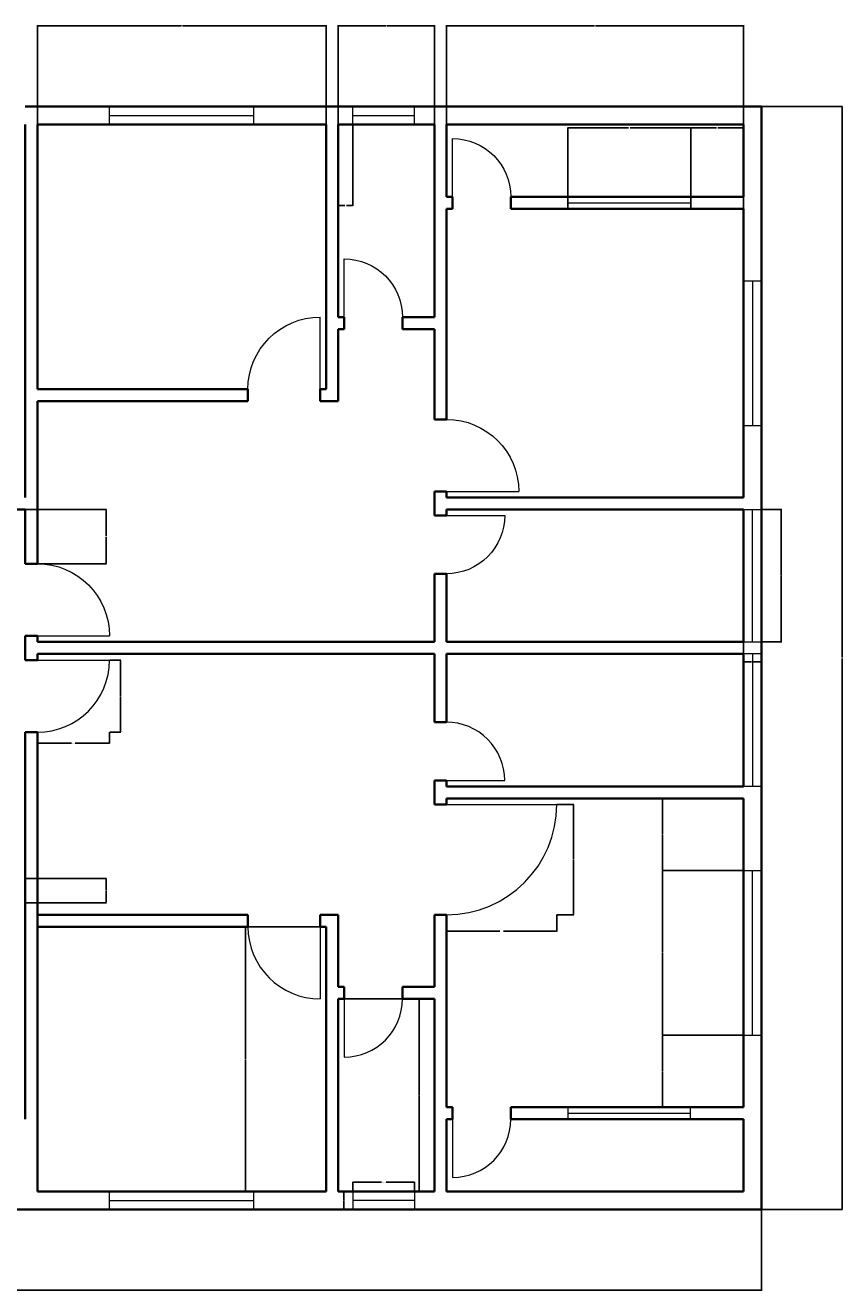
# Model space of a CAD drawing. Units: inches. Extents: x 2811 to 3694, y 2039 to 2670.
# Tile 3 of 3: x 3286 to 3694, y 2039 to 2670. Entities that reach past the tile are written whole.
import ezdxf

# ---------------------------------------------------------------- set-up
doc = ezdxf.new("R2010")
doc.units = ezdxf.units.IN
for name, color, linetype, lineweight in [('A-ANNO-DIMS', 2, 'Continuous', 18), ('A-DOOR', 3, 'Continuous', 18), ('A-GLAZ', 4, 'Continuous', 18), ('A-WALL', 7, 'Continuous', 35)]:
    doc.layers.add(name, color=color, linetype=linetype, lineweight=lineweight)
doc.styles.get("Standard").update_dxf_attribs({"font": 'arial.ttf'})
doc.dimstyles.get("Standard").update_dxf_attribs({"dimtxt": 0.18, "dimasz": 0.18, "dimexe": 0.18, "dimexo": 0.0625, "dimgap": 0.09, "dimtad": 0, "dimtih": 1, "dimtoh": 1, "dimdec": 4, "dimzin": 0, "dimdsep": 46, "dimtxsty": 'Standard', "dimcen": 0.09, "dimadec": 0, "dimazin": 0, "dimtfac": 1, "dimtdec": 4, "dimtofl": 0, "dimtmove": 0, "dimatfit": 3, "dimfxl": 1, "dimtolj": 1, "dimtzin": 0, "dimarcsym": 0})

# ---------------------------------------------------------------- blocks, each defined once
blk = doc.blocks.new('DOOR-SWING-29IN')
blk.add_line((29, 0), (29, 29))
blk.add_arc((29, 0), 29, 90, 180)
blk = doc.blocks.new('DOOR-SWING-36IN')
blk.add_line((36, 0), (0, 0))
blk.add_arc((36, 0), 36, 90, 180)
blk = doc.blocks.new('DOOR-SWING-55IN')
blk.add_line((0, 55), (55, 55))
blk.add_arc((0, 55), 55, 270, 0)
blk = doc.blocks.new('WIN-72IN')
for p, q in [((0, 0), (0, 9)), ((72, 0), (72, 9)), ((0, 4.5), (72, 4.5))]:
    blk.add_line(p, q)
blk = doc.blocks.new('WIN-66IN')
for p, q in [((0, 66), (9, 66)), ((4.5, 0), (4.5, 66)), ((0, 0), (9, 0))]:
    blk.add_line(p, q)
blk = doc.blocks.new('WIN-30_67IN')
for p, q in [((0, 0), (0, 9)), ((30.67, 0), (30.67, 9)), ((0, 4.5), (30.67, 4.5))]:
    blk.add_line(p, q)
blk = doc.blocks.new('*D10')
at = {"layer": 'A-ANNO-DIMS', "color": 0, "lineweight": -2, "transparency": 16777216}
for p, q in [((3292.28, 2317.92), (3292.28, 2312.4)), ((3328.28, 2317.92), (3328.28, 2312.4)), ((3292.46, 2312.58), (3309.34, 2312.58)), ((3328.1, 2312.58), (3311.21, 2312.58))]:
    blk.add_line(p, q, dxfattribs=at)
at = {"layer": 'A-ANNO-DIMS', "color": 0, "transparency": 16777216}
for points in [[(3292.46, 2312.61), (3292.46, 2312.55), (3292.28, 2312.58)], [(3328.1, 2312.61), (3328.1, 2312.55), (3328.28, 2312.58)]]:
    blk.add_solid(points, dxfattribs=at)
at = {"layer": 'Defpoints', "color": 0, "transparency": 16777216}
for p in [(3292.28, 2317.98), (3328.28, 2317.98), (3292.28, 2312.58)]:
    blk.add_point(p, dxfattribs=at)
at = {"layer": 'A-ANNO-DIMS', "color": 0, "transparency": 16777216, "insert": (3310.28, 2312.58), "char_height": 0.18, "attachment_point": 5}
blk.add_mtext('\\A1;DOOR 36 TYP.', dxfattribs=at)
blk = doc.blocks.new('*D11')
at = {"layer": 'A-ANNO-DIMS', "color": 0, "lineweight": -2, "transparency": 16777216}
for p, q in [((3328.34, 2353.98), (3333.86, 2353.98)), ((3333.68, 2353.8), (3333.68, 2336.16)), ((3333.68, 2318.16), (3333.68, 2335.8)), ((3328.34, 2317.98), (3333.86, 2317.98))]:
    blk.add_line(p, q, dxfattribs=at)
at = {"layer": 'A-ANNO-DIMS', "color": 0, "transparency": 16777216}
for points in [[(3333.65, 2353.8), (3333.71, 2353.8), (3333.68, 2353.98)], [(3333.65, 2318.16), (3333.71, 2318.16), (3333.68, 2317.98)]]:
    blk.add_solid(points, dxfattribs=at)
at = {"layer": 'Defpoints', "color": 0, "transparency": 16777216}
for p in [(3328.28, 2353.98), (3328.28, 2317.98), (3333.68, 2317.98)]:
    blk.add_point(p, dxfattribs=at)
at = {"layer": 'A-ANNO-DIMS', "color": 0, "transparency": 16777216, "insert": (3333.68, 2335.98), "char_height": 0.18, "attachment_point": 5}
blk.add_mtext('\\A1;36 TYP.', dxfattribs=at)
blk = doc.blocks.new('*D12')
at = {"layer": 'A-ANNO-DIMS', "color": 0, "lineweight": -2, "transparency": 16777216}
for p, q in [((3496.28, 2226.92), (3496.28, 2218.55)), ((3551.28, 2226.92), (3551.28, 2218.55)), ((3496.46, 2218.73), (3522.84, 2218.73)), ((3551.1, 2218.73), (3524.71, 2218.73))]:
    blk.add_line(p, q, dxfattribs=at)
at = {"layer": 'A-ANNO-DIMS', "color": 0, "transparency": 16777216}
for points in [[(3496.46, 2218.76), (3496.46, 2218.7), (3496.28, 2218.73)], [(3551.1, 2218.76), (3551.1, 2218.7), (3551.28, 2218.73)]]:
    blk.add_solid(points, dxfattribs=at)
at = {"layer": 'Defpoints', "color": 0, "transparency": 16777216}
for p in [(3496.28, 2226.98), (3551.28, 2226.98), (3551.28, 2218.73)]:
    blk.add_point(p, dxfattribs=at)
at = {"layer": 'A-ANNO-DIMS', "color": 0, "transparency": 16777216, "insert": (3523.78, 2218.73), "char_height": 0.18, "attachment_point": 5}
blk.add_mtext('\\A1;DOOR 55 TYP.', dxfattribs=at)
blk = doc.blocks.new('*D13')
at = {"layer": 'A-ANNO-DIMS', "color": 0, "lineweight": -2, "transparency": 16777216}
for p, q in [((3551.34, 2281.98), (3559.71, 2281.98)), ((3559.53, 2281.8), (3559.53, 2254.66)), ((3559.53, 2227.16), (3559.53, 2254.3)), ((3551.34, 2226.98), (3559.71, 2226.98))]:
    blk.add_line(p, q, dxfattribs=at)
at = {"layer": 'A-ANNO-DIMS', "color": 0, "transparency": 16777216}
for points in [[(3559.5, 2281.8), (3559.56, 2281.8), (3559.53, 2281.98)], [(3559.5, 2227.16), (3559.56, 2227.16), (3559.53, 2226.98)]]:
    blk.add_solid(points, dxfattribs=at)
at = {"layer": 'Defpoints', "color": 0, "transparency": 16777216}
for p in [(3551.28, 2281.98), (3559.53, 2281.98), (3551.28, 2226.98)]:
    blk.add_point(p, dxfattribs=at)
at = {"layer": 'A-ANNO-DIMS', "color": 0, "transparency": 16777216, "insert": (3559.53, 2254.48), "char_height": 0.18, "attachment_point": 5}
blk.add_mtext('\\A1;55 TYP.', dxfattribs=at)
blk = doc.blocks.new('*D16')
at = {"layer": 'A-ANNO-DIMS', "color": 0, "lineweight": -2, "transparency": 16777216}
for p, q in [((3653.34, 2428.98), (3663.36, 2428.98)), ((3663.18, 2428.8), (3663.18, 2396.16)), ((3663.18, 2363.16), (3663.18, 2395.8)), ((3653.34, 2362.98), (3663.36, 2362.98))]:
    blk.add_line(p, q, dxfattribs=at)
at = {"layer": 'A-ANNO-DIMS', "color": 0, "transparency": 16777216}
for points in [[(3663.15, 2428.8), (3663.21, 2428.8), (3663.18, 2428.98)], [(3663.15, 2363.16), (3663.21, 2363.16), (3663.18, 2362.98)]]:
    blk.add_solid(points, dxfattribs=at)
at = {"layer": 'Defpoints', "color": 0, "transparency": 16777216}
for p in [(3653.28, 2428.98), (3663.18, 2428.98), (3653.28, 2362.98)]:
    blk.add_point(p, dxfattribs=at)
at = {"layer": 'A-ANNO-DIMS', "color": 0, "transparency": 16777216, "insert": (3663.18, 2395.98), "char_height": 0.18, "attachment_point": 5}
blk.add_mtext('\\A1;WINDOW 66 TYP.', dxfattribs=at)
blk = doc.blocks.new('*D17')
at = {"layer": 'A-ANNO-DIMS', "color": 0, "lineweight": -2, "transparency": 16777216}
for p, q in [((3644.28, 2362.92), (3644.28, 2352.9)), ((3653.28, 2362.92), (3653.28, 2352.9)), ((3644.46, 2353.08), (3648.32, 2353.08)), ((3653.1, 2353.08), (3649.23, 2353.08))]:
    blk.add_line(p, q, dxfattribs=at)
at = {"layer": 'A-ANNO-DIMS', "color": 0, "transparency": 16777216}
for points in [[(3644.46, 2353.11), (3644.46, 2353.05), (3644.28, 2353.08)], [(3653.1, 2353.11), (3653.1, 2353.05), (3653.28, 2353.08)]]:
    blk.add_solid(points, dxfattribs=at)
at = {"layer": 'Defpoints', "color": 0, "transparency": 16777216}
for p in [(3644.28, 2362.98), (3653.28, 2362.98), (3653.28, 2353.08)]:
    blk.add_point(p, dxfattribs=at)
at = {"layer": 'A-ANNO-DIMS', "color": 0, "transparency": 16777216, "insert": (3648.78, 2353.08), "char_height": 0.18, "attachment_point": 5}
blk.add_mtext('\\A1;9 TYP.', dxfattribs=at)
blk = doc.blocks.new('*D20')
at = {"layer": 'A-ANNO-DIMS', "color": 0, "lineweight": -2, "transparency": 16777216}
for p, q in [((3449.64, 2089.04), (3449.64, 2093.76)), ((3449.82, 2093.58), (3463.86, 2093.58)), ((3480.13, 2093.58), (3466.1, 2093.58)), ((3480.31, 2089.04), (3480.31, 2093.76))]:
    blk.add_line(p, q, dxfattribs=at)
at = {"layer": 'A-ANNO-DIMS', "color": 0, "transparency": 16777216}
for points in [[(3449.82, 2093.61), (3449.82, 2093.55), (3449.64, 2093.58)], [(3480.13, 2093.61), (3480.13, 2093.55), (3480.31, 2093.58)]]:
    blk.add_solid(points, dxfattribs=at)
at = {"layer": 'Defpoints', "color": 0, "transparency": 16777216}
for p in [(3449.64, 2093.58), (3449.64, 2088.98), (3480.31, 2088.98)]:
    blk.add_point(p, dxfattribs=at)
at = {"layer": 'A-ANNO-DIMS', "color": 0, "transparency": 16777216, "insert": (3464.98, 2093.58), "char_height": 0.18, "attachment_point": 5}
blk.add_mtext('\\A1;WINDOW 31 TYP.', dxfattribs=at)
blk = doc.blocks.new('*D21')
at = {"layer": 'A-ANNO-DIMS', "color": 0, "lineweight": -2, "transparency": 16777216}
for p, q in [((3449.58, 2088.98), (3444.86, 2088.98)), ((3445.04, 2088.8), (3445.04, 2084.66)), ((3445.04, 2080.16), (3445.04, 2084.3)), ((3449.58, 2079.98), (3444.86, 2079.98))]:
    blk.add_line(p, q, dxfattribs=at)
at = {"layer": 'A-ANNO-DIMS', "color": 0, "transparency": 16777216}
for points in [[(3445.01, 2088.8), (3445.07, 2088.8), (3445.04, 2088.98)], [(3445.01, 2080.16), (3445.07, 2080.16), (3445.04, 2079.98)]]:
    blk.add_solid(points, dxfattribs=at)
at = {"layer": 'Defpoints', "color": 0, "transparency": 16777216}
for p in [(3449.64, 2088.98), (3445.04, 2079.98), (3449.64, 2079.98)]:
    blk.add_point(p, dxfattribs=at)
at = {"layer": 'A-ANNO-DIMS', "color": 0, "transparency": 16777216, "insert": (3445.04, 2084.48), "char_height": 0.18, "attachment_point": 5}
blk.add_mtext('\\A1;9 TYP.', dxfattribs=at)
blk = doc.blocks.new('*D22')
at = {"layer": 'A-ANNO-DIMS', "color": 0, "lineweight": -2, "transparency": 16777216}
for p, q in [((2851.28, 2079.92), (2851.28, 2039.5)), ((3653.28, 2079.92), (3653.28, 2039.5)), ((2851.46, 2039.68), (3251.99, 2039.68)), ((3653.1, 2039.68), (3252.56, 2039.68))]:
    blk.add_line(p, q, dxfattribs=at)
at = {"layer": 'A-ANNO-DIMS', "color": 0, "transparency": 16777216}
for points in [[(2851.46, 2039.71), (2851.46, 2039.65), (2851.28, 2039.68)], [(3653.1, 2039.71), (3653.1, 2039.65), (3653.28, 2039.68)]]:
    blk.add_solid(points, dxfattribs=at)
at = {"layer": 'Defpoints', "color": 0, "transparency": 16777216}
for p in [(2851.28, 2079.98), (3653.28, 2079.98), (3653.28, 2039.68)]:
    blk.add_point(p, dxfattribs=at)
at = {"layer": 'A-ANNO-DIMS', "color": 0, "transparency": 16777216, "insert": (3252.28, 2039.68), "char_height": 0.18, "attachment_point": 5}
blk.add_mtext('\\A1;802', dxfattribs=at)
blk = doc.blocks.new('*D23')
at = {"layer": 'A-ANNO-DIMS', "color": 0, "lineweight": -2, "transparency": 16777216}
for p, q in [((3653.34, 2629.98), (3693.76, 2629.98)), ((3693.58, 2629.8), (3693.58, 2355.16)), ((3693.58, 2080.16), (3693.58, 2354.8)), ((3653.34, 2079.98), (3693.76, 2079.98))]:
    blk.add_line(p, q, dxfattribs=at)
at = {"layer": 'A-ANNO-DIMS', "color": 0, "transparency": 16777216}
for points in [[(3693.55, 2629.8), (3693.61, 2629.8), (3693.58, 2629.98)], [(3693.55, 2080.16), (3693.61, 2080.16), (3693.58, 2079.98)]]:
    blk.add_solid(points, dxfattribs=at)
at = {"layer": 'Defpoints', "color": 0, "transparency": 16777216}
for p in [(3653.28, 2629.98), (3693.58, 2629.98), (3653.28, 2079.98)]:
    blk.add_point(p, dxfattribs=at)
at = {"layer": 'A-ANNO-DIMS', "color": 0, "transparency": 16777216, "insert": (3693.58, 2354.98), "char_height": 0.18, "attachment_point": 5}
blk.add_mtext('\\A1;550', dxfattribs=at)
blk = doc.blocks.new('*D28')
at = {"layer": 'A-ANNO-DIMS', "color": 0, "lineweight": -2, "transparency": 16777216}
for p, q in [((3292.28, 2621.04), (3292.28, 2670.46)), ((3292.46, 2670.28), (3364, 2670.28)), ((3436.1, 2670.28), (3364.56, 2670.28)), ((3436.28, 2621.04), (3436.28, 2670.46))]:
    blk.add_line(p, q, dxfattribs=at)
at = {"layer": 'A-ANNO-DIMS', "color": 0, "transparency": 16777216}
for points in [[(3292.46, 2670.31), (3292.46, 2670.25), (3292.28, 2670.28)], [(3436.1, 2670.31), (3436.1, 2670.25), (3436.28, 2670.28)]]:
    blk.add_solid(points, dxfattribs=at)
at = {"layer": 'Defpoints', "color": 0, "transparency": 16777216}
for p in [(3436.28, 2670.28), (3292.28, 2620.98), (3436.28, 2620.98)]:
    blk.add_point(p, dxfattribs=at)
at = {"layer": 'A-ANNO-DIMS', "color": 0, "transparency": 16777216, "insert": (3364.28, 2670.28), "char_height": 0.18, "attachment_point": 5}
blk.add_mtext('\\A1;144', dxfattribs=at)
blk = doc.blocks.new('*D29')
at = {"layer": 'A-ANNO-DIMS', "color": 0, "lineweight": -2, "transparency": 16777216}
for p, q in [((3442.28, 2621.04), (3442.28, 2670.46)), ((3442.46, 2670.28), (3466.05, 2670.28)), ((3490.1, 2670.28), (3466.5, 2670.28)), ((3490.28, 2621.04), (3490.28, 2670.46))]:
    blk.add_line(p, q, dxfattribs=at)
at = {"layer": 'A-ANNO-DIMS', "color": 0, "transparency": 16777216}
for points in [[(3442.46, 2670.31), (3442.46, 2670.25), (3442.28, 2670.28)], [(3490.1, 2670.31), (3490.1, 2670.25), (3490.28, 2670.28)]]:
    blk.add_solid(points, dxfattribs=at)
at = {"layer": 'Defpoints', "color": 0, "transparency": 16777216}
for p in [(3490.28, 2670.28), (3442.28, 2620.98), (3490.28, 2620.98)]:
    blk.add_point(p, dxfattribs=at)
at = {"layer": 'A-ANNO-DIMS', "color": 0, "transparency": 16777216, "insert": (3466.28, 2670.28), "char_height": 0.18, "attachment_point": 5}
blk.add_mtext('\\A1;48', dxfattribs=at)
blk = doc.blocks.new('*D30')
at = {"layer": 'A-ANNO-DIMS', "color": 0, "lineweight": -2, "transparency": 16777216}
for p, q in [((3496.28, 2621.04), (3496.28, 2670.46)), ((3496.46, 2670.28), (3570, 2670.28)), ((3644.1, 2670.28), (3570.56, 2670.28)), ((3644.28, 2621.04), (3644.28, 2670.46))]:
    blk.add_line(p, q, dxfattribs=at)
at = {"layer": 'A-ANNO-DIMS', "color": 0, "transparency": 16777216}
for points in [[(3496.46, 2670.31), (3496.46, 2670.25), (3496.28, 2670.28)], [(3644.1, 2670.31), (3644.1, 2670.25), (3644.28, 2670.28)]]:
    blk.add_solid(points, dxfattribs=at)
at = {"layer": 'Defpoints', "color": 0, "transparency": 16777216}
for p in [(3644.28, 2670.28), (3496.28, 2620.98), (3644.28, 2620.98)]:
    blk.add_point(p, dxfattribs=at)
at = {"layer": 'A-ANNO-DIMS', "color": 0, "transparency": 16777216, "insert": (3570.28, 2670.28), "char_height": 0.18, "attachment_point": 5}
blk.add_mtext('\\A1;148', dxfattribs=at)
blk = doc.blocks.new('*D42')
at = {"layer": 'A-ANNO-DIMS', "color": 0, "lineweight": -2, "transparency": 16777216}
for p, q in [((3436.21, 2220.98), (3395.8, 2220.98)), ((3395.98, 2220.8), (3395.98, 2155.16)), ((3395.98, 2089.16), (3395.98, 2154.8)), ((3436.21, 2088.98), (3395.8, 2088.98))]:
    blk.add_line(p, q, dxfattribs=at)
at = {"layer": 'A-ANNO-DIMS', "color": 0, "transparency": 16777216}
for points in [[(3395.95, 2220.8), (3396.01, 2220.8), (3395.98, 2220.98)], [(3395.95, 2089.16), (3396.01, 2089.16), (3395.98, 2088.98)]]:
    blk.add_solid(points, dxfattribs=at)
at = {"layer": 'Defpoints', "color": 0, "transparency": 16777216}
for p in [(3395.98, 2220.98), (3436.28, 2220.98), (3436.28, 2088.98)]:
    blk.add_point(p, dxfattribs=at)
at = {"layer": 'A-ANNO-DIMS', "color": 0, "transparency": 16777216, "insert": (3395.98, 2154.98), "char_height": 0.18, "attachment_point": 5}
blk.add_mtext('\\A1;132', dxfattribs=at)
blk = doc.blocks.new('*D43')
at = {"layer": 'A-ANNO-DIMS', "color": 0, "lineweight": -2, "transparency": 16777216}
for p, q in [((3442.34, 2184.98), (3482.76, 2184.98)), ((3482.58, 2184.8), (3482.58, 2137.16)), ((3482.58, 2089.16), (3482.58, 2136.8)), ((3442.34, 2088.98), (3482.76, 2088.98))]:
    blk.add_line(p, q, dxfattribs=at)
at = {"layer": 'A-ANNO-DIMS', "color": 0, "transparency": 16777216}
for points in [[(3482.55, 2184.8), (3482.61, 2184.8), (3482.58, 2184.98)], [(3482.55, 2089.16), (3482.61, 2089.16), (3482.58, 2088.98)]]:
    blk.add_solid(points, dxfattribs=at)
at = {"layer": 'Defpoints', "color": 0, "transparency": 16777216}
for p in [(3442.28, 2184.98), (3442.28, 2088.98), (3482.58, 2088.98)]:
    blk.add_point(p, dxfattribs=at)
at = {"layer": 'A-ANNO-DIMS', "color": 0, "transparency": 16777216, "insert": (3482.58, 2136.98), "char_height": 0.18, "attachment_point": 5}
blk.add_mtext('\\A1;96', dxfattribs=at)
blk = doc.blocks.new('*D44')
at = {"layer": 'A-ANNO-DIMS', "color": 0, "lineweight": -2, "transparency": 16777216}
for p, q in [((3644.21, 2248.98), (3603.8, 2248.98)), ((3603.98, 2248.8), (3603.98, 2208.16)), ((3603.98, 2167.16), (3603.98, 2207.8)), ((3644.21, 2166.98), (3603.8, 2166.98))]:
    blk.add_line(p, q, dxfattribs=at)
at = {"layer": 'A-ANNO-DIMS', "color": 0, "transparency": 16777216}
for points in [[(3603.95, 2248.8), (3604.01, 2248.8), (3603.98, 2248.98)], [(3603.95, 2167.16), (3604.01, 2167.16), (3603.98, 2166.98)]]:
    blk.add_solid(points, dxfattribs=at)
at = {"layer": 'Defpoints', "color": 0, "transparency": 16777216}
for p in [(3603.98, 2248.98), (3644.28, 2248.98), (3644.28, 2166.98)]:
    blk.add_point(p, dxfattribs=at)
at = {"layer": 'A-ANNO-DIMS', "color": 0, "transparency": 16777216, "insert": (3603.98, 2207.98), "char_height": 0.18, "attachment_point": 5}
blk.add_mtext('\\A1;82', dxfattribs=at)
blk = doc.blocks.new('*D45')
at = {"layer": 'A-ANNO-DIMS', "color": 0, "lineweight": -2, "transparency": 16777216}
for p, q in [((3644.21, 2166.98), (3603.8, 2166.98)), ((3603.98, 2166.8), (3603.98, 2149.16)), ((3603.98, 2131.16), (3603.98, 2148.8)), ((3644.21, 2130.98), (3603.8, 2130.98))]:
    blk.add_line(p, q, dxfattribs=at)
at = {"layer": 'A-ANNO-DIMS', "color": 0, "transparency": 16777216}
for points in [[(3603.95, 2166.8), (3604.01, 2166.8), (3603.98, 2166.98)], [(3603.95, 2131.16), (3604.01, 2131.16), (3603.98, 2130.98)]]:
    blk.add_solid(points, dxfattribs=at)
at = {"layer": 'Defpoints', "color": 0, "transparency": 16777216}
for p in [(3603.98, 2166.98), (3644.28, 2166.98), (3644.28, 2130.98)]:
    blk.add_point(p, dxfattribs=at)
at = {"layer": 'A-ANNO-DIMS', "color": 0, "transparency": 16777216, "insert": (3603.98, 2148.98), "char_height": 0.18, "attachment_point": 5}
blk.add_mtext('\\A1;36', dxfattribs=at)
blk = doc.blocks.new('*D46')
at = {"layer": 'A-ANNO-DIMS', "color": 0, "lineweight": -2, "transparency": 16777216}
for p, q in [((3644.21, 2284.98), (3603.8, 2284.98)), ((3603.98, 2284.8), (3603.98, 2267.16)), ((3603.98, 2249.16), (3603.98, 2266.8)), ((3644.21, 2248.98), (3603.8, 2248.98))]:
    blk.add_line(p, q, dxfattribs=at)
at = {"layer": 'A-ANNO-DIMS', "color": 0, "transparency": 16777216}
for points in [[(3603.95, 2284.8), (3604.01, 2284.8), (3603.98, 2284.98)], [(3603.95, 2249.16), (3604.01, 2249.16), (3603.98, 2248.98)]]:
    blk.add_solid(points, dxfattribs=at)
at = {"layer": 'Defpoints', "color": 0, "transparency": 16777216}
for p in [(3603.98, 2284.98), (3644.28, 2284.98), (3644.28, 2248.98)]:
    blk.add_point(p, dxfattribs=at)
at = {"layer": 'A-ANNO-DIMS', "color": 0, "transparency": 16777216, "insert": (3603.98, 2266.98), "char_height": 0.18, "attachment_point": 5}
blk.add_mtext('\\A1;36', dxfattribs=at)
blk = doc.blocks.new('*D49')
at = {"layer": 'A-ANNO-DIMS', "color": 0, "lineweight": -2, "transparency": 16777216}
for p, q in [((3556.69, 2579.04), (3556.69, 2619.46)), ((3556.87, 2619.28), (3587.02, 2619.28)), ((3617.96, 2619.28), (3587.81, 2619.28)), ((3618.14, 2579.04), (3618.14, 2619.46))]:
    blk.add_line(p, q, dxfattribs=at)
at = {"layer": 'A-ANNO-DIMS', "color": 0, "transparency": 16777216}
for points in [[(3556.87, 2619.31), (3556.87, 2619.25), (3556.69, 2619.28)], [(3617.96, 2619.31), (3617.96, 2619.25), (3618.14, 2619.28)]]:
    blk.add_solid(points, dxfattribs=at)
at = {"layer": 'Defpoints', "color": 0, "transparency": 16777216}
for p in [(3618.14, 2619.28), (3556.69, 2578.98), (3618.14, 2578.98)]:
    blk.add_point(p, dxfattribs=at)
at = {"layer": 'A-ANNO-DIMS', "color": 0, "transparency": 16777216, "insert": (3587.42, 2619.28), "char_height": 0.18, "attachment_point": 5}
blk.add_mtext('\\A1;61.46', dxfattribs=at)
blk = doc.blocks.new('*D50')
at = {"layer": 'A-ANNO-DIMS', "color": 0, "lineweight": -2, "transparency": 16777216}
for p, q in [((3618.14, 2579.04), (3618.14, 2619.46)), ((3618.32, 2619.28), (3630.82, 2619.28)), ((3644.1, 2619.28), (3631.61, 2619.28)), ((3644.28, 2579.04), (3644.28, 2619.46))]:
    blk.add_line(p, q, dxfattribs=at)
at = {"layer": 'A-ANNO-DIMS', "color": 0, "transparency": 16777216}
for points in [[(3618.32, 2619.31), (3618.32, 2619.25), (3618.14, 2619.28)], [(3644.1, 2619.31), (3644.1, 2619.25), (3644.28, 2619.28)]]:
    blk.add_solid(points, dxfattribs=at)
at = {"layer": 'Defpoints', "color": 0, "transparency": 16777216}
for p in [(3644.28, 2619.28), (3618.14, 2578.98), (3644.28, 2578.98)]:
    blk.add_point(p, dxfattribs=at)
at = {"layer": 'A-ANNO-DIMS', "color": 0, "transparency": 16777216, "insert": (3631.21, 2619.28), "char_height": 0.18, "attachment_point": 5}
blk.add_mtext('\\A1;26.13', dxfattribs=at)
blk = doc.blocks.new('*D53')
at = {"layer": 'A-ANNO-DIMS', "color": 0, "lineweight": -2, "transparency": 16777216}
for p, q in [((3442.28, 2620.92), (3442.28, 2580.5)), ((3449.64, 2620.92), (3449.64, 2580.5)), ((3442.46, 2580.68), (3445.57, 2580.68)), ((3449.46, 2580.68), (3446.35, 2580.68))]:
    blk.add_line(p, q, dxfattribs=at)
at = {"layer": 'A-ANNO-DIMS', "color": 0, "transparency": 16777216}
for points in [[(3442.46, 2580.71), (3442.46, 2580.65), (3442.28, 2580.68)], [(3449.46, 2580.71), (3449.46, 2580.65), (3449.64, 2580.68)]]:
    blk.add_solid(points, dxfattribs=at)
at = {"layer": 'Defpoints', "color": 0, "transparency": 16777216}
for p in [(3442.28, 2620.98), (3449.64, 2620.98), (3442.28, 2580.68)]:
    blk.add_point(p, dxfattribs=at)
at = {"layer": 'A-ANNO-DIMS', "color": 0, "transparency": 16777216, "insert": (3445.96, 2580.68), "char_height": 0.18, "attachment_point": 5}
blk.add_mtext('\\A1;7.364', dxfattribs=at)
blk = doc.blocks.new('*D57')
at = {"layer": 'A-ANNO-DIMS', "color": 0, "lineweight": -2, "transparency": 16777216}
for p, q in [((3286.34, 2244.98), (3326.76, 2244.98)), ((3326.58, 2244.8), (3326.58, 2239.16)), ((3326.58, 2233.16), (3326.58, 2238.8)), ((3286.34, 2232.98), (3326.76, 2232.98))]:
    blk.add_line(p, q, dxfattribs=at)
at = {"layer": 'A-ANNO-DIMS', "color": 0, "transparency": 16777216}
for points in [[(3326.55, 2244.8), (3326.61, 2244.8), (3326.58, 2244.98)], [(3326.55, 2233.16), (3326.61, 2233.16), (3326.58, 2232.98)]]:
    blk.add_solid(points, dxfattribs=at)
at = {"layer": 'Defpoints', "color": 0, "transparency": 16777216}
for p in [(3286.28, 2244.98), (3286.28, 2232.98), (3326.58, 2232.98)]:
    blk.add_point(p, dxfattribs=at)
at = {"layer": 'A-ANNO-DIMS', "color": 0, "transparency": 16777216, "insert": (3326.58, 2238.98), "char_height": 0.18, "attachment_point": 5}
blk.add_mtext('\\A1;12', dxfattribs=at)
blk = doc.blocks.new('*D60')
at = {"layer": 'A-ANNO-DIMS', "color": 0, "lineweight": -2, "transparency": 16777216}
for p, q in [((3286.34, 2428.98), (3326.76, 2428.98)), ((3326.58, 2428.8), (3326.58, 2415.66)), ((3326.58, 2402.16), (3326.58, 2415.3)), ((3286.34, 2401.98), (3326.76, 2401.98))]:
    blk.add_line(p, q, dxfattribs=at)
at = {"layer": 'A-ANNO-DIMS', "color": 0, "transparency": 16777216}
for points in [[(3326.55, 2428.8), (3326.61, 2428.8), (3326.58, 2428.98)], [(3326.55, 2402.16), (3326.61, 2402.16), (3326.58, 2401.98)]]:
    blk.add_solid(points, dxfattribs=at)
at = {"layer": 'Defpoints', "color": 0, "transparency": 16777216}
for p in [(3286.28, 2428.98), (3286.28, 2401.98), (3326.58, 2401.98)]:
    blk.add_point(p, dxfattribs=at)
at = {"layer": 'A-ANNO-DIMS', "color": 0, "transparency": 16777216, "insert": (3326.58, 2415.48), "char_height": 0.18, "attachment_point": 5}
blk.add_mtext('\\A1;27', dxfattribs=at)

msp = doc.modelspace()

# ---------------------------------------------------------------- linework, layer by layer
at = {"layer": 'A-GLAZ'}
for p, q in [((3556.6891, 2584.9792), (3556.6891, 2578.9792)), ((3556.6891, 2581.9792), (3618.1446, 2581.9792)), ((3618.1446, 2584.9792), (3618.1446, 2578.9792)), ((3644.2765, 2248.9792), (3653.2765, 2248.9792)), ((3648.7765, 2166.9792), (3648.7765, 2248.9792)), ((3644.2765, 2166.9792), (3653.2765, 2166.9792)), ((3556.6891, 2130.9792), (3556.6891, 2124.9792)), ((3556.6891, 2127.9792), (3617.6891, 2127.9792)), ((3617.6891, 2130.9792), (3617.6891, 2124.9792)), ((3328.2765, 2079.9792), (3400.2765, 2079.9792))]:
    msp.add_line(p, q, dxfattribs=at)
at = {"layer": 'A-WALL'}
for p, q in [((3653.2765, 2629.9792), (3286.2765, 2629.9792)), ((3653.2765, 2124.9792), (3653.2765, 2629.9792)), ((3286.2765, 2620.9792), (3286.2765, 2434.9792)), ((3292.2765, 2620.9792), (3292.2765, 2488.9792)), ((3436.2765, 2620.9792), (3292.2765, 2620.9792)), ((3436.2765, 2620.9792), (3436.2765, 2488.9792)), ((3442.2765, 2620.9792), (3442.2765, 2524.9792)), ((3490.2765, 2620.9792), (3442.2765, 2620.9792)), ((3490.2765, 2620.9792), (3490.2765, 2524.9792)), ((3644.2765, 2620.9792), (3496.2765, 2620.9792)), ((3496.2765, 2620.9792), (3496.2765, 2584.9792)), ((3644.2765, 2584.9792), (3644.2765, 2620.9792)), ((3499.2765, 2584.9792), (3496.2765, 2584.9792)), ((3499.2765, 2584.9792), (3499.2765, 2578.9792)), ((3644.2765, 2584.9792), (3528.2765, 2584.9792)), ((3528.2765, 2584.9792), (3528.2765, 2578.9792)), ((3496.2765, 2578.9792), (3496.2765, 2473.9792)), ((3499.2765, 2578.9792), (3496.2765, 2578.9792)), ((3644.2765, 2578.9792), (3528.2765, 2578.9792)), ((3644.2765, 2434.9792), (3644.2765, 2578.9792)), ((3445.2765, 2524.9792), (3442.2765, 2524.9792)), ((3445.2765, 2524.9792), (3445.2765, 2518.9792)), ((3490.2765, 2524.9792), (3474.2765, 2524.9792)), ((3474.2765, 2524.9792), (3474.2765, 2518.9792)), ((3442.2765, 2518.9792), (3442.2765, 2482.9792)), ((3445.2765, 2518.9792), (3442.2765, 2518.9792)), ((3490.2765, 2518.9792), (3474.2765, 2518.9792)), ((3490.2765, 2518.9792), (3490.2765, 2473.9792)), ((3397.2765, 2488.9792), (3292.2765, 2488.9792)), ((3397.2765, 2488.9792), (3397.2765, 2482.9792)), ((3436.2765, 2488.9792), (3433.2765, 2488.9792)), ((3433.2765, 2488.9792), (3433.2765, 2482.9792)), ((3292.2765, 2482.9792), (3292.2765, 2401.9792)), ((3397.2765, 2482.9792), (3292.2765, 2482.9792)), ((3436.2765, 2482.9792), (3433.2765, 2482.9792)), ((3436.2765, 2482.9792), (3442.2765, 2482.9792)), ((3496.2765, 2473.9792), (3490.2765, 2473.9792)), ((3496.2765, 2437.9792), (3490.2765, 2437.9792)), ((3490.2765, 2437.9792), (3490.2765, 2425.9792)), ((3496.2765, 2437.9792), (3496.2765, 2434.9792)), ((3644.2765, 2434.9792), (3496.2765, 2434.9792)), ((3286.2765, 2428.9792), (3214.2765, 2428.9792)), ((3286.2765, 2428.9792), (3286.2765, 2401.9792)), ((3496.2765, 2425.9792), (3490.2765, 2425.9792)), ((3644.2765, 2428.9792), (3496.2765, 2428.9792)), ((3496.2765, 2428.9792), (3496.2765, 2425.9792)), ((3644.2765, 2362.9792), (3644.2765, 2428.9792)), ((3292.2765, 2401.9792), (3286.2765, 2401.9792)), ((3496.2765, 2396.9792), (3490.2765, 2396.9792)), ((3490.2765, 2396.9792), (3490.2765, 2362.9792)), ((3496.2765, 2396.9792), (3496.2765, 2362.9792)), ((3292.2765, 2365.9792), (3286.2765, 2365.9792)), ((3286.2765, 2365.9792), (3286.2765, 2353.9792)), ((3292.2765, 2365.9792), (3292.2765, 2362.9792)), ((3490.2765, 2362.9792), (3292.2765, 2362.9792)), ((3644.2765, 2362.9792), (3496.2765, 2362.9792)), ((3292.2765, 2353.9792), (3286.2765, 2353.9792)), ((3490.2765, 2356.9792), (3292.2765, 2356.9792)), ((3292.2765, 2356.9792), (3292.2765, 2353.9792)), ((3490.2765, 2356.9792), (3490.2765, 2322.9792)), ((3644.2765, 2356.9792), (3496.2765, 2356.9792)), ((3496.2765, 2356.9792), (3496.2765, 2322.9792)), ((3644.2765, 2290.9792), (3644.2765, 2356.9792)), ((3496.2765, 2322.9792), (3490.2765, 2322.9792)), ((3292.2765, 2317.9792), (3286.2765, 2317.9792)), ((3286.2765, 2317.9792), (3286.2765, 2133.9792)), ((3292.2765, 2317.9792), (3292.2765, 2271.9792)), ((3496.2765, 2293.9792), (3490.2765, 2293.9792)), ((3490.2765, 2293.9792), (3490.2765, 2281.9792)), ((3496.2765, 2293.9792), (3496.2765, 2290.9792)), ((3644.2765, 2290.9792), (3496.2765, 2290.9792)), ((3644.2765, 2284.9792), (3496.2765, 2284.9792)), ((3496.2765, 2284.9792), (3496.2765, 2281.9792)), ((3644.2765, 2175.9792), (3644.2765, 2284.9792)), ((3496.2765, 2281.9792), (3490.2765, 2281.9792)), ((3292.2765, 2271.9792), (3292.2765, 2265.9792)), ((3292.2765, 2265.9792), (3292.2765, 2133.9792)), ((3292.2765, 2226.9792), (3397.2765, 2226.9792)), ((3292.2765, 2220.9792), (3397.2765, 2220.9792)), ((3397.2765, 2220.9792), (3397.2765, 2226.9792)), ((3433.2765, 2220.9792), (3433.2765, 2226.9792)), ((3433.2765, 2226.9792), (3436.2765, 2226.9792)), ((3433.2765, 2220.9792), (3436.2765, 2220.9792)), ((3436.2765, 2226.9792), (3442.2765, 2226.9792)), ((3436.2765, 2220.9792), (3436.2765, 2133.9792)), ((3442.2765, 2226.9792), (3442.2765, 2190.9792)), ((3490.2765, 2226.9792), (3490.2765, 2190.9792)), ((3490.2765, 2226.9792), (3496.2765, 2226.9792)), ((3496.2765, 2226.9792), (3496.2765, 2175.9792)), ((3644.2765, 2130.9792), (3644.2765, 2198.0155)), ((3442.2765, 2190.9792), (3445.2765, 2190.9792)), ((3445.2765, 2190.9792), (3445.2765, 2184.9792)), ((3474.2765, 2190.9792), (3474.2765, 2184.9792)), ((3474.2765, 2190.9792), (3490.2765, 2190.9792)), ((3442.2765, 2184.9792), (3445.2765, 2184.9792)), ((3442.2765, 2184.9792), (3442.2765, 2133.9792)), ((3474.2765, 2184.9792), (3490.2765, 2184.9792)), ((3490.2765, 2184.9792), (3490.2765, 2133.9792)), ((3496.2765, 2175.9792), (3496.2765, 2169.9792)), ((3496.2765, 2169.9792), (3496.2765, 2133.9792)), ((3644.2765, 2133.9792), (3644.2765, 2169.9792)), ((3286.2765, 2133.9792), (3286.2765, 2124.9792)), ((3292.2765, 2088.9792), (3292.2765, 2133.9792)), ((3436.2765, 2133.9792), (3436.2765, 2088.9792)), ((3442.2765, 2088.9792), (3442.2765, 2133.9792)), ((3490.2765, 2133.9792), (3490.2765, 2088.9792)), ((3496.2765, 2133.9792), (3496.2765, 2130.9792)), ((3496.2765, 2130.9792), (3499.2765, 2130.9792)), ((3499.2765, 2130.9792), (3499.2765, 2124.9792)), ((3528.2765, 2130.9792), (3528.2765, 2124.9792)), ((3528.2765, 2130.9792), (3644.2765, 2130.9792)), ((3496.2765, 2088.9792), (3496.2765, 2124.9792)), ((3496.2765, 2124.9792), (3499.2765, 2124.9792)), ((3528.2765, 2124.9792), (3644.2765, 2124.9792)), ((3644.2765, 2124.9792), (3644.2765, 2088.9792)), ((3653.2765, 2124.9792), (3653.2765, 2079.9792)), ((3292.2765, 2088.9792), (3436.2765, 2088.9792)), ((3442.2765, 2088.9792), (3490.2765, 2088.9792)), ((3496.2765, 2088.9792), (3644.2765, 2088.9792)), ((2851.2765, 2079.9792), (3653.2765, 2079.9792))]:
    msp.add_line(p, q, dxfattribs=at)

# ---------------------------------------------------------------- block references
at = {"layer": 'A-DOOR', "extrusion": (0, 0, -1), "zscale": -1}
for name, p in [('DOOR-SWING-29IN', (-3528.2761, 2584.979)), ('DOOR-SWING-29IN', (-3474.2761, 2524.979)), ('DOOR-SWING-36IN', (-3532.2761, 2437.979)), ('DOOR-SWING-36IN', (-3328.2761, 2365.979))]:
    msp.add_blockref(name, p, dxfattribs=at)
for name, p, rotation in [('DOOR-SWING-36IN', (-3433.2768, 2524.9788), 269.9999999999997), ('DOOR-SWING-29IN', (-3496.2763, 2396.9797), 89.99999999999999)]:
    msp.add_blockref(name, p, dxfattribs=dict(at, rotation=rotation))
at = {"layer": 'A-DOOR'}
for name, p, rotation in [('DOOR-SWING-36IN', (3328.2761, 2353.9795), 180), ('DOOR-SWING-29IN', (3496.2763, 2322.9788), 270.0000000000009), ('DOOR-SWING-36IN', (3433.2768, 2184.9797), 90), ('DOOR-SWING-29IN', (3474.2761, 2184.9795), 180), ('DOOR-SWING-29IN', (3528.2761, 2124.9795), 180)]:
    msp.add_blockref(name, p, dxfattribs=dict(at, rotation=rotation))
msp.add_blockref('DOOR-SWING-55IN', (3496.277, 2226.979), dxfattribs=at)
at = {"layer": 'A-GLAZ'}
for name, p in [('WIN-72IN', (3328.277, 2620.979)), ('WIN-30_67IN', (3449.64, 2620.979)), ('WIN-66IN', (3644.277, 2362.979)), ('WIN-72IN', (3328.277, 2079.979))]:
    msp.add_blockref(name, p, dxfattribs=at)
for name, p, rotation in [('WIN-72IN', (3644.2763, 2542.9788), 269.9999999999987), ('WIN-66IN', (3653.2761, 2356.9795), 180), ('WIN-30_67IN', (3480.3144, 2088.9795), 180)]:
    msp.add_blockref(name, p, dxfattribs=dict(at, rotation=rotation))

# ---------------------------------------------------------------- dimensions: what is measured, and where the dimension line sits
at = {"layer": 'A-ANNO-DIMS'}
for base, p1, p2, override, picture, middle in [((3436.2765, 2670.2792), (3292.2765, 2620.9792), (3436.2765, 2620.9792), {"dimdec": 0, "dimlfac": 1, "dimrnd": 0, "dimzin": 0, "dimdsep": 46, "dimlunit": 2}, '*D28', (3364.2765, 2670.2792)), ((3490.2765, 2670.2792), (3442.2765, 2620.9792), (3490.2765, 2620.9792), {"dimdec": 0, "dimlfac": 1, "dimrnd": 0, "dimzin": 0, "dimdsep": 46, "dimlunit": 2}, '*D29', (3466.2765, 2670.2792)), ((3644.2765, 2670.2792), (3496.2765, 2620.9792), (3644.2765, 2620.9792), {"dimdec": 0, "dimlfac": 1, "dimrnd": 0, "dimzin": 0, "dimdsep": 46, "dimlunit": 2}, '*D30', (3570.2765, 2670.2792)), ((3618.1446, 2619.2792), (3556.6891, 2578.9792), (3618.1446, 2578.9792), {"dimdec": 2, "dimlfac": 1, "dimrnd": 0, "dimzin": 0, "dimdsep": 46, "dimlunit": 2}, '*D49', (3587.4169, 2619.2792)), ((3653.2765, 2039.6792), (2851.2765, 2079.9792), (3653.2765, 2079.9792), {"dimdec": 0, "dimlfac": 1, "dimrnd": 0, "dimzin": 0, "dimdsep": 46, "dimlunit": 2}, '*D22', (3252.2765, 2039.6792))]:
    dim = msp.add_linear_dim(base=base, p1=p1, p2=p2, dimstyle='Standard', override=override, dxfattribs=at)
    dim.commit()
    dim.dimension.update_dxf_attribs({"geometry": picture, "text_midpoint": middle})
for base, p1, p2, angle, override, picture, middle in [((3693.5765, 2629.9792), (3653.2765, 2079.9792), (3653.2765, 2629.9792), 90, {"dimdec": 0, "dimlfac": 1, "dimrnd": 0, "dimzin": 0, "dimdsep": 46, "dimlunit": 2}, '*D23', (3693.5765, 2354.9792)), ((3442.2765, 2580.6792), (3449.6403, 2620.9792), (3442.2765, 2620.9792), 180, {"dimdec": 3, "dimlfac": 1, "dimrnd": 0, "dimzin": 0, "dimdsep": 46, "dimlunit": 2}, '*D53', (3445.9584, 2580.6792)), ((3644.2765, 2619.2792), (3618.1446, 2578.9792), (3644.2765, 2578.9792), 0, {"dimdec": 2, "dimlfac": 1, "dimrnd": 0, "dimzin": 0, "dimdsep": 46, "dimlunit": 2}, '*D50', (3631.2106, 2619.2792)), ((3326.5765, 2401.9792), (3286.2765, 2428.9792), (3286.2765, 2401.9792), 270, {"dimdec": 0, "dimlfac": 1, "dimrnd": 0, "dimzin": 0, "dimdsep": 46, "dimlunit": 2}, '*D60', (3326.5765, 2415.4792)), ((3603.9765, 2284.9792), (3644.2765, 2248.9792), (3644.2765, 2284.9792), 90, {"dimdec": 0, "dimlfac": 1, "dimrnd": 0, "dimzin": 0, "dimdsep": 46, "dimlunit": 2}, '*D46', (3603.9765, 2266.9792)), ((3603.9765, 2248.9792), (3644.2765, 2166.9792), (3644.2765, 2248.9792), 90, {"dimdec": 0, "dimlfac": 1, "dimrnd": 0, "dimzin": 0, "dimdsep": 46, "dimlunit": 2}, '*D44', (3603.9765, 2207.9792)), ((3326.5765, 2232.9792), (3286.2765, 2244.9792), (3286.2765, 2232.9792), 270, {"dimdec": 0, "dimlfac": 1, "dimrnd": 0, "dimzin": 0, "dimdsep": 46, "dimlunit": 2}, '*D57', (3326.5765, 2238.9792)), ((3395.9765, 2220.9792), (3436.2765, 2088.9792), (3436.2765, 2220.9792), 90, {"dimdec": 0, "dimlfac": 1, "dimrnd": 0, "dimzin": 0, "dimdsep": 46, "dimlunit": 2}, '*D42', (3395.9765, 2154.9792)), ((3482.5765, 2088.9792), (3442.2765, 2184.9792), (3442.2765, 2088.9792), 270, {"dimdec": 0, "dimlfac": 1, "dimrnd": 0, "dimzin": 0, "dimdsep": 46, "dimlunit": 2}, '*D43', (3482.5765, 2136.9792)), ((3603.9765, 2166.9792), (3644.2765, 2130.9792), (3644.2765, 2166.9792), 90, {"dimdec": 0, "dimlfac": 1, "dimrnd": 0, "dimzin": 0, "dimdsep": 46, "dimlunit": 2}, '*D45', (3603.9765, 2148.9792))]:
    dim = msp.add_linear_dim(base=base, p1=p1, p2=p2, angle=angle, dimstyle='Standard', override=override, dxfattribs=at)
    dim.commit()
    dim.dimension.update_dxf_attribs({"geometry": picture, "text_midpoint": middle})
for base, p1, p2, angle, text, picture, middle in [((3663.1765, 2428.9792), (3653.2765, 2362.9792), (3653.2765, 2428.9792), 90, 'WINDOW <> TYP.', '*D16', (3663.1765, 2395.9792)), ((3333.6765, 2317.9792), (3328.2765, 2353.9792), (3328.2765, 2317.9792), 270, '<> TYP.', '*D11', (3333.6765, 2335.9792)), ((3292.2765, 2312.5792), (3328.2765, 2317.9792), (3292.2765, 2317.9792), 180, 'DOOR <> TYP.', '*D10', (3310.2765, 2312.5792)), ((3559.5265, 2281.9792), (3551.2765, 2226.9792), (3551.2765, 2281.9792), 90, '<> TYP.', '*D13', (3559.5265, 2254.4792)), ((3445.0392, 2079.9792), (3449.6403, 2088.9792), (3449.6403, 2079.9792), 270, '<> TYP.', '*D21', (3445.0392, 2084.4792)), ((3449.6403, 2093.5803), (3480.3141, 2088.9792), (3449.6403, 2088.9792), 180, 'WINDOW <> TYP.', '*D20', (3464.9772, 2093.5803))]:
    dim = msp.add_linear_dim(base=base, p1=p1, p2=p2, angle=angle, text=text, dimstyle='Standard', override={"dimdec": 0, "dimlfac": 1, "dimrnd": 0, "dimzin": 0, "dimdsep": 46, "dimlunit": 2}, dxfattribs=at)
    dim.commit()
    dim.dimension.update_dxf_attribs({"geometry": picture, "text_midpoint": middle})
for base, p1, p2, text, picture, middle in [((3653.2765, 2353.0792), (3644.2765, 2362.9792), (3653.2765, 2362.9792), '<> TYP.', '*D17', (3648.7765, 2353.0792)), ((3551.2765, 2218.7292), (3496.2765, 2226.9792), (3551.2765, 2226.9792), 'DOOR <> TYP.', '*D12', (3523.7765, 2218.7292))]:
    dim = msp.add_linear_dim(base=base, p1=p1, p2=p2, text=text, dimstyle='Standard', override={"dimdec": 0, "dimlfac": 1, "dimrnd": 0, "dimzin": 0, "dimdsep": 46, "dimlunit": 2}, dxfattribs=at)
    dim.commit()
    dim.dimension.update_dxf_attribs({"geometry": picture, "text_midpoint": middle})

doc.saveas('drawing.dxf')
